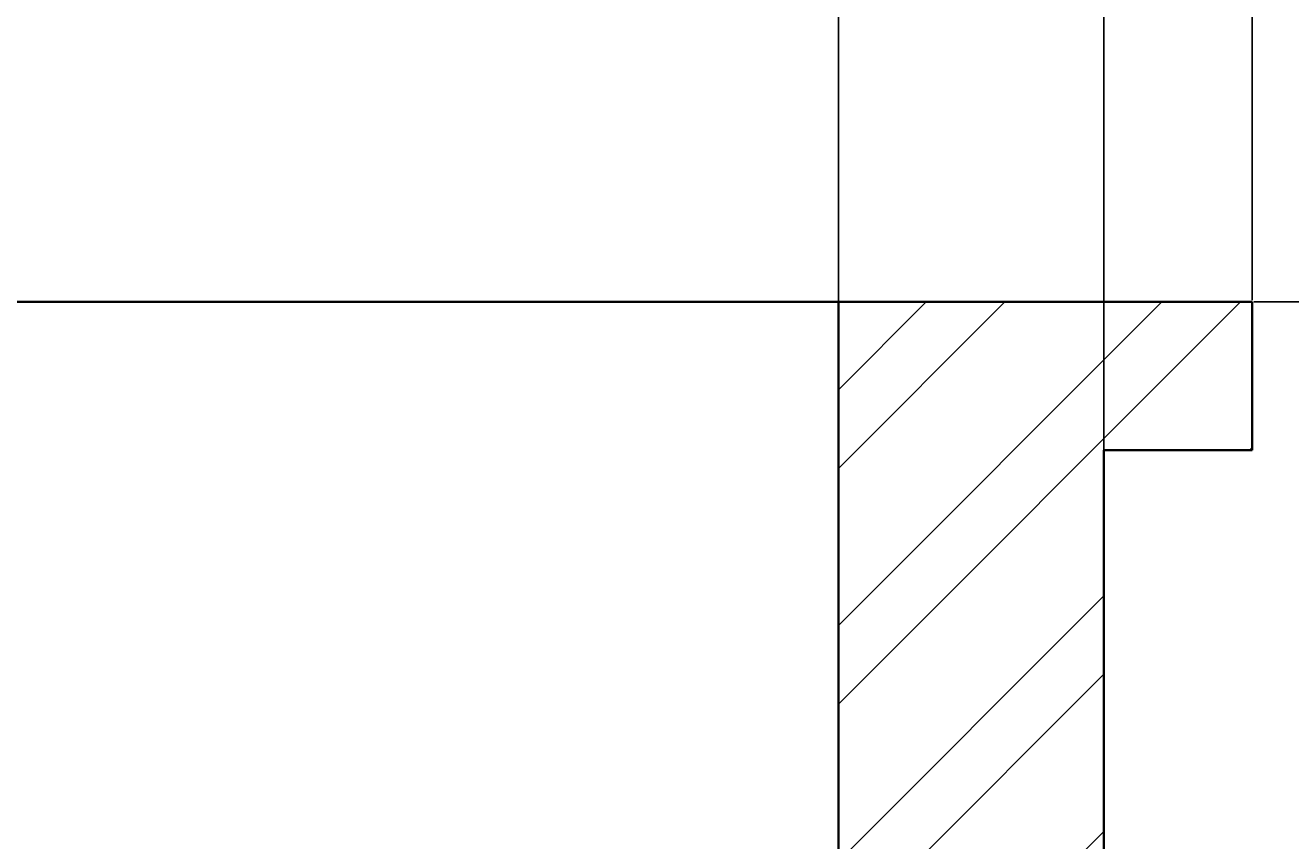
# Model space of a CAD drawing. Units: inches. Extents: x -301 to 715, y -607 to 364.
# Tile 49 of 141: x 107 to 150, y -343 to -315. Entities that reach past the tile are written whole.
import ezdxf

# ---------------------------------------------------------------- set-up
doc = ezdxf.new("R2010")
doc.units = ezdxf.units.IN
doc.header["$MEASUREMENT"] = 0
for name, color, linetype, lineweight in [('A-ANNO-DIMS', 2, 'Continuous', 18), ('A-SECT', 1, 'Continuous', 35), ('A-SECT-PATT', 8, 'Continuous', 13)]:
    doc.layers.add(name, color=color, linetype=linetype, lineweight=lineweight)
doc.styles.get("Standard").update_dxf_attribs({"font": 'arial.ttf'})
doc.dimstyles.get("Standard").update_dxf_attribs({"dimtxt": 0.18, "dimasz": 0.18, "dimexe": 0.18, "dimexo": 0.0625, "dimgap": 0.09, "dimtad": 0, "dimtih": 1, "dimtoh": 1, "dimdec": 1, "dimzin": 0, "dimdsep": 46, "dimlunit": 4, "dimtxsty": 'Standard', "dimcen": 0.09, "dimclrd": 3, "dimclre": 4, "dimclrt": 6, "dimadec": 0, "dimazin": 0, "dimtfac": 1, "dimtdec": 1, "dimtofl": 0, "dimtmove": 0, "dimatfit": 3, "dimfxl": 1, "dimtfill": 2, "dimtfillclr": 51, "dimtolj": 1, "dimtzin": 0, "dimarcsym": 0})

# ---------------------------------------------------------------- blocks, each defined once
blk = doc.blocks.new('*D175')
at = {"layer": 'A-ANNO-DIMS', "color": 4, "lineweight": -2, "transparency": 16777216}
for p, q in [((-199.282, -324.415), (-199.282, -292.467)), ((148.218, -324.415), (148.218, -292.467))]:
    blk.add_line(p, q, dxfattribs=at)
at = {"layer": 'A-ANNO-DIMS', "color": 3, "lineweight": -2, "transparency": 16777216}
for p, q in [((-199.102, -292.647), (-26.212, -292.647)), ((148.038, -292.647), (-24.852, -292.647))]:
    blk.add_line(p, q, dxfattribs=at)
at = {"layer": 'A-ANNO-DIMS', "color": 3, "transparency": 16777216}
for points in [[(-199.102, -292.617), (-199.102, -292.677), (-199.282, -292.647)], [(148.038, -292.617), (148.038, -292.677), (148.218, -292.647)]]:
    blk.add_solid(points, dxfattribs=at)
at = {"layer": 'Defpoints', "color": 0, "transparency": 16777216}
for p in [(148.218, -292.647), (-199.282, -324.477), (148.218, -324.477)]:
    blk.add_point(p, dxfattribs=at)
at = {"layer": 'A-ANNO-DIMS', "color": 6, "transparency": 16777216, "insert": (-25.532, -292.647), "char_height": 0.18, "attachment_point": 5, "bg_fill": 1, "box_fill_scale": 1.25, "bg_fill_color": 51, "bg_fill_transparency": 0}
blk.add_mtext('\\A1;28\'-11 1/2"', dxfattribs=at)
blk = doc.blocks.new('*D176')
at = {"layer": 'A-ANNO-DIMS', "color": 4, "lineweight": -2, "transparency": 16777216}
for p, q in [((148.28, -324.477), (215.605, -324.477)), ((-15.22, -540.477), (215.605, -540.477))]:
    blk.add_line(p, q, dxfattribs=at)
at = {"layer": 'A-ANNO-DIMS', "color": 3, "lineweight": -2, "transparency": 16777216}
for p, q in [((215.425, -324.657), (215.425, -432.296)), ((215.425, -540.297), (215.425, -432.659))]:
    blk.add_line(p, q, dxfattribs=at)
at = {"layer": 'A-ANNO-DIMS', "color": 3, "transparency": 16777216}
for points in [[(215.395, -324.657), (215.455, -324.657), (215.425, -324.477)], [(215.395, -540.297), (215.455, -540.297), (215.425, -540.477)]]:
    blk.add_solid(points, dxfattribs=at)
at = {"layer": 'Defpoints', "color": 0, "transparency": 16777216}
for p in [(148.218, -324.477), (-15.282, -540.477), (215.425, -540.477)]:
    blk.add_point(p, dxfattribs=at)
at = {"layer": 'A-ANNO-DIMS', "color": 6, "transparency": 16777216, "insert": (215.425, -432.477), "char_height": 0.18, "attachment_point": 5, "bg_fill": 1, "box_fill_scale": 1.25, "bg_fill_color": 51, "bg_fill_transparency": 0}
blk.add_mtext('\\A1;18\'-0"', dxfattribs=at)
blk = doc.blocks.new('*D186')
at = {"layer": 'A-ANNO-DIMS', "color": 4, "lineweight": -2, "transparency": 16777216}
for p, q in [((134.255, -353.415), (134.255, -292.467)), ((143.218, -353.415), (143.218, -292.467))]:
    blk.add_line(p, q, dxfattribs=at)
at = {"layer": 'A-ANNO-DIMS', "color": 3, "lineweight": -2, "transparency": 16777216}
for p, q in [((134.435, -292.647), (138.407, -292.647)), ((143.038, -292.647), (139.066, -292.647))]:
    blk.add_line(p, q, dxfattribs=at)
at = {"layer": 'A-ANNO-DIMS', "color": 3, "transparency": 16777216}
for points in [[(134.435, -292.617), (134.435, -292.677), (134.255, -292.647)], [(143.038, -292.617), (143.038, -292.677), (143.218, -292.647)]]:
    blk.add_solid(points, dxfattribs=at)
at = {"layer": 'Defpoints', "color": 0, "transparency": 16777216}
for p in [(143.218, -292.647), (134.255, -353.477), (143.218, -353.477)]:
    blk.add_point(p, dxfattribs=at)
at = {"layer": 'A-ANNO-DIMS', "color": 6, "transparency": 16777216, "insert": (138.737, -292.647), "char_height": 0.18, "attachment_point": 5, "bg_fill": 1, "box_fill_scale": 1.25, "bg_fill_color": 51, "bg_fill_transparency": 0}
blk.add_mtext('\\A1;0\'-9"', dxfattribs=at)

msp = doc.modelspace()

# ---------------------------------------------------------------- hatches: boundary and pattern name
at = {"layer": 'A-SECT-PATT'}
h = msp.add_hatch(dxfattribs=at)
h.set_pattern_fill('ANSI32', color=256, scale=15)
h.set_pattern_definition([(45, (10.321, 33.8764), (-3.977476, 3.977476), []), (45, (12.973, 33.8764), (-3.977476, 3.977476), [])])
h.paths.add_polyline_path([(-185.282, -324.477), (-199.282, -324.477), (-199.282, -329.477), (-194.282, -329.477), (-194.282, -353.477), (-185.282, -353.477)])
h.paths.add_polyline_path([(-185.282, -361.477), (-193.904, -361.477), (-193.982, -377.537), (-185.282, -377.537)])
h.paths.add_polyline_path([(143.218, -329.477), (148.218, -329.477), (148.218, -324.477), (134.255, -324.477), (134.255, -353.477), (143.218, -353.477)])
h.paths.add_polyline_path([(143.218, -361.477), (134.255, -361.477), (134.255, -377.477), (143.218, -377.477)])
h.paths.add_polyline_path([(-185.282, -439.477), (-194.282, -439.477), (-194.282, -463.477), (-185.282, -463.477)])
h.paths.add_polyline_path([(-185.282, -471.477), (-194.282, -471.477), (-194.282, -481.477), (-185.282, -481.477)])
h.paths.add_polyline_path([(-185.282, -463.477), (-194.282, -463.477), (-194.282, -466.477), (-185.282, -466.477)])
h.paths.add_polyline_path([(-185.282, -466.477), (-194.282, -466.477), (-194.282, -471.477), (-185.282, -471.477)])
h.paths.add_polyline_path([(-180.282, -481.477), (-185.282, -481.477), (-194.282, -481.477), (-199.282, -481.477), (-199.282, -493.477), (-180.282, -493.477)])
h.paths.add_polyline_path([(-175.282, -493.477), (-180.282, -493.477), (-199.282, -493.477), (-204.282, -493.477), (-204.282, -511.477), (-175.282, -511.477)])
h.paths.add_polyline_path([(-170.282, -511.477), (-175.282, -511.477), (-204.282, -511.477), (-209.282, -511.477), (-209.282, -535.477), (-170.282, -535.477)])
h.paths.add_polyline_path([(-35.282, -463.477), (-41.282, -463.477), (-41.282, -466.477), (-35.282, -466.477)])
h.paths.add_polyline_path([(-35.282, -466.477), (-41.282, -466.477), (-41.282, -471.477), (-35.282, -471.477)])
h.paths.add_polyline_path([(-35.282, -471.477), (-41.282, -471.477), (-41.282, -481.477), (-35.282, -481.477)])
h.paths.add_polyline_path([(-30.282, -481.477), (-46.282, -481.477), (-46.282, -493.477), (-30.282, -493.477)])
h.paths.add_polyline_path([(-25.282, -493.477), (-30.282, -493.477), (-46.282, -493.477), (-51.282, -493.477), (-51.282, -511.477), (-25.282, -511.477)])
h.paths.add_polyline_path([(-20.282, -511.477), (-25.282, -511.477), (-51.282, -511.477), (-56.282, -511.477), (-56.282, -535.477), (-20.282, -535.477)])
h.paths.add_polyline_path([(143.218, -463.477), (134.255, -463.477), (134.255, -466.477), (143.218, -466.477)])
h.paths.add_polyline_path([(143.218, -466.477), (134.255, -466.477), (134.255, -471.477), (143.218, -471.477)])
h.paths.add_polyline_path([(143.218, -471.477), (134.255, -471.477), (134.255, -481.477), (143.218, -481.477)])
h.paths.add_polyline_path([(148.255, -481.477), (143.255, -481.477), (134.255, -481.477), (129.255, -481.477), (129.255, -493.477), (148.255, -493.477)])
h.paths.add_polyline_path([(153.255, -493.477), (148.255, -493.477), (129.255, -493.477), (124.255, -493.477), (124.255, -511.477), (153.255, -511.477)])
h.paths.add_polyline_path([(158.255, -511.477), (153.255, -511.477), (124.255, -511.477), (119.255, -511.477), (119.255, -535.477), (158.255, -535.477)])

# ---------------------------------------------------------------- linework, layer by layer
at = {"layer": 'A-SECT'}
for p, q in [((-185.282, -324.477), (134.255, -324.477)), ((148.218, -324.477), (134.255, -324.477)), ((134.255, -324.477), (134.255, -353.477)), ((148.218, -329.477), (148.218, -324.477)), ((143.218, -353.477), (143.218, -329.477)), ((143.218, -329.477), (148.218, -329.477))]:
    msp.add_line(p, q, dxfattribs=at)

# ---------------------------------------------------------------- dimensions: what is measured, and where the dimension line sits
at = {"layer": 'A-ANNO-DIMS'}
for base, p1, p2, picture, middle in [((148.218, -292.647), (-199.282, -324.477), (148.218, -324.477), '*D175', (-25.532, -292.647)), ((143.218, -292.647), (134.255, -353.477), (143.218, -353.477), '*D186', (138.737, -292.647))]:
    dim = msp.add_linear_dim(base=base, p1=p1, p2=p2, dimstyle='Standard', override={"dimdec": 1, "dimlfac": 1, "dimrnd": 0, "dimzin": 1, "dimdsep": 46, "dimlunit": 4, "dimfrac": 2}, dxfattribs=at)
    dim.commit()
    dim.dimension.update_dxf_attribs({"geometry": picture, "text_midpoint": middle})
dim = msp.add_linear_dim(base=(215.425, -540.477), p1=(148.218, -324.477), p2=(-15.282, -540.477), angle=90, dimstyle='Standard', override={"dimdec": 1, "dimlfac": 1, "dimrnd": 0, "dimzin": 1, "dimdsep": 46, "dimlunit": 4, "dimfrac": 2}, dxfattribs=at)
dim.commit()
dim.dimension.update_dxf_attribs({"geometry": '*D176', "text_midpoint": (215.425, -432.477)})

doc.saveas('drawing.dxf')
